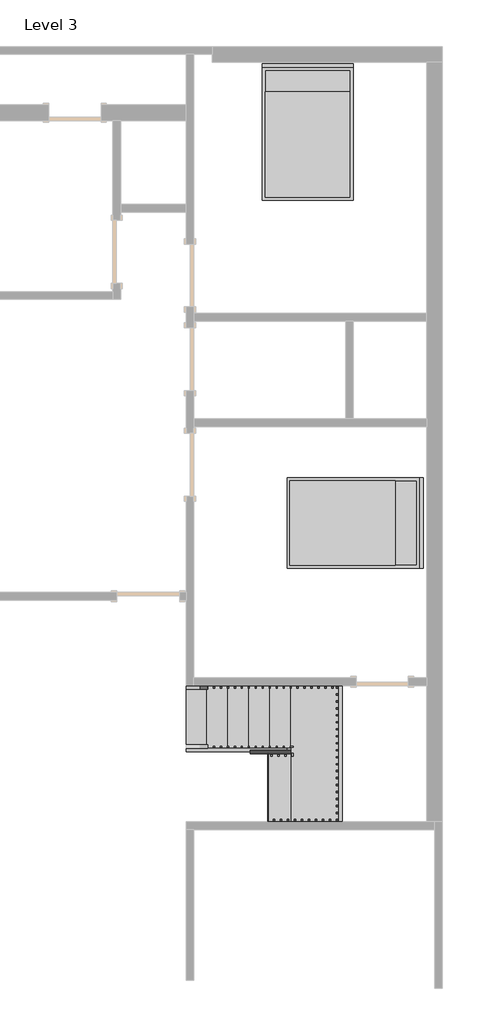
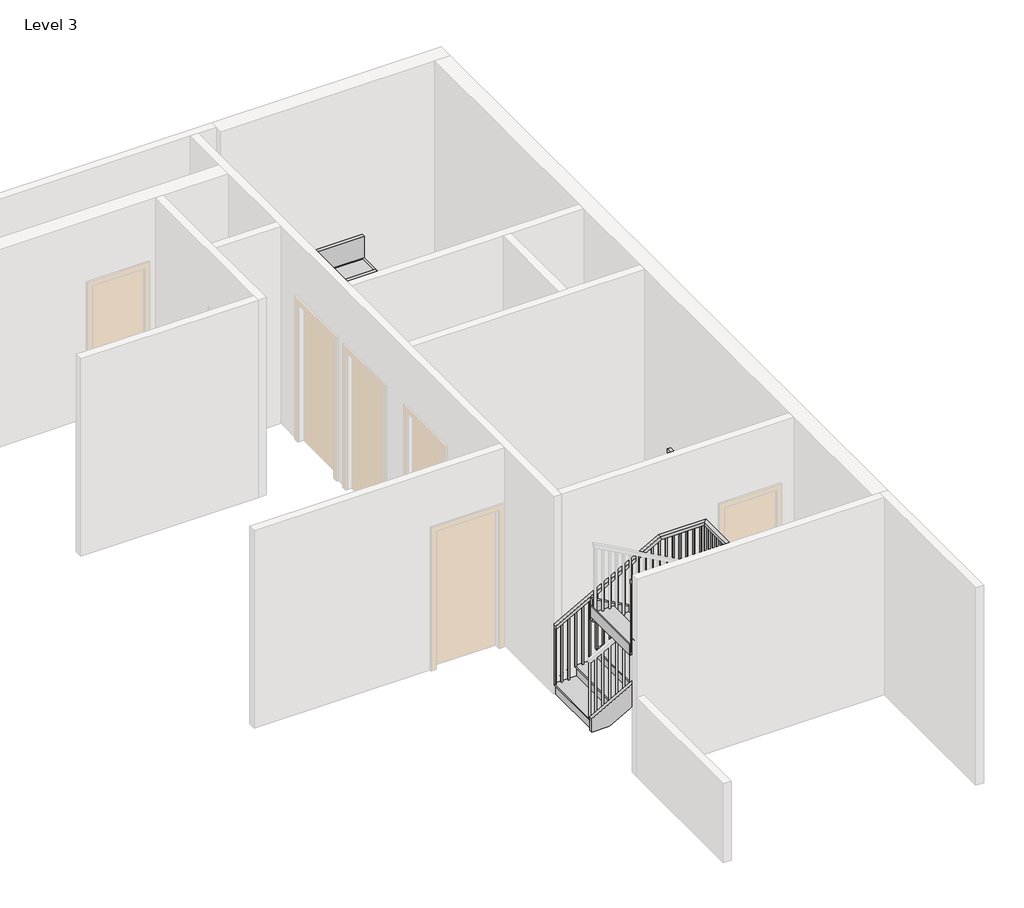
# One storey, part 2 of 2: 6 members, 2 furniture elements, 1 railing, 1 stair flight.
"""IFC4 building model written with IfcOpenShell, lengths in millimetres."""

from ifc_helpers import new_model, si_unit, frame, origin, place, context, project, spatial, polyline, outline, extrude, faceted_brep, transform, mapped, element, save
from components import bed_17739_bed_17739_15c61121, stair_flight_96a85028

model = new_model("IFC4")

# Units and contexts
model_context = context("Model", 3, world=origin())
ifc_project = project(units=[si_unit("LENGTHUNIT", "METRE", prefix="MILLI")], contexts=[model_context])

# Site, building, storey
site = spatial("IfcSite", under=ifc_project)
building = spatial("IfcBuilding", under=site)
storey = spatial("IfcBuildingStorey", under=building, Name="Level 3", Elevation=3200.4)

# Furniture
placement = place(None, origin())
bed_17739_bed_17739_shape = bed_17739_bed_17739_15c61121(model_context)
element("IfcFurniture", 1, ObjectType="Bed_17739 : Bed_17739", at=placement, inside=storey, context=model_context, shape_type="MappedRepresentation", body=[
    mapped(bed_17739_bed_17739_shape, transform((592.6084916, 6126.1935985, 3200.4), x_axis=(1.0, 0.0, 0.0), y_axis=(0.0, 1.0, 0.0), z_axis=(0.0, 0.0, 1.0))),
])
element("IfcFurniture", 2, ObjectType="Bed_17739 : Bed_17739", at=placement, inside=storey, context=model_context, shape_type="MappedRepresentation", body=[
    mapped(bed_17739_bed_17739_shape, transform((1259.3584916, 455.6435985, 3200.4), x_axis=(0.0, -1.0, 0.0), y_axis=(1.0, 0.0, 0.0), z_axis=(0.0, 0.0, 1.0))),
])

# Members
element("IfcMember", 3, ObjectType="Stringer - 2\" Width", at=placement, inside=storey, context=model_context, shape_type="SweptSolid", body=[
    extrude(outline(polyline([(3407.9983948, -1179.0415084), (3200.4, -1179.0415084), (3200.4, -925.0970056), (4292.6, 1040.8629944), (4292.6, 413.241381), (3407.9983948, -1179.0415084)])), frame((0.0, -1912.9064015, 0.0), z_axis=(0.0, 1.0, 0.0), x_axis=(0.0, 0.0, 1.0)), (0.0, 0.0, 1.0), 50.8),
])
element("IfcMember", 4, ObjectType="Stringer - 2\" Width", at=placement, inside=storey, context=model_context, shape_type="SweptSolid", body=[
    extrude(outline(polyline([(1043.4584916, -1862.1064015), (1094.2584916, -1862.1064015), (1094.2584916, -3894.1064015), (1043.4584916, -3894.1064015), (1043.4584916, -1862.1064015)])), frame((0.0, 0.0, 3987.8), z_axis=(0.0, 0.0, 1.0), x_axis=(1.0, 0.0, 0.0)), (0.0, 0.0, 1.0), 304.8),
])
element("IfcMember", 5, ObjectType="Stringer - 2\" Width", at=placement, inside=storey, context=model_context, shape_type="SweptSolid", body=[
    extrude(outline(polyline([(3987.8, 1094.2584916), (4007.720617, 1094.2584916), (5270.6650614, -1179.0415084), (4921.9863873, -1179.0415084), (3987.8, 502.4939888), (3987.8, 1094.2584916)])), frame((0.0, -3944.9064015, 0.0), z_axis=(0.0, 1.0, 0.0), x_axis=(0.0, 0.0, 1.0)), (0.0, 0.0, 1.0), 50.8),
])
element("IfcMember", 6, ObjectType="Stringer - 2\" Width", at=placement, inside=storey, context=model_context, shape_type="SweptSolid", body=[
    extrude(outline(polyline([(3407.9983948, -1179.0415084), (3200.4, -1179.0415084), (3200.4, -925.0970056), (3877.7641651, 294.1584916), (4226.4428392, 294.1584916), (3407.9983948, -1179.0415084)])), frame((0.0, -2878.1064015, 0.0), z_axis=(0.0, 1.0, 0.0), x_axis=(0.0, 0.0, 1.0)), (0.0, 0.0, 1.0), 50.8),
])
element("IfcMember", 7, ObjectType="Stringer - 2\" Width", at=placement, inside=storey, context=model_context, shape_type="SweptSolid", body=[
    extrude(outline(polyline([(294.1584916, -2827.3064015), (344.9584916, -2827.3064015), (344.9584916, -2852.7064015), (294.1584916, -2852.7064015), (294.1584916, -2827.3064015)])), frame((0.0, 0.0, 3987.8), z_axis=(0.0, 0.0, 1.0), x_axis=(1.0, 0.0, 0.0)), (0.0, 0.0, 1.0), 304.8),
])
element("IfcMember", 8, ObjectType="Stringer - 2\" Width", at=placement, inside=storey, context=model_context, shape_type="SweptSolid", body=[
    extrude(outline(polyline([(4075.3197207, 344.9584916), (4423.9983948, 344.9584916), (5270.6650614, -1179.0415084), (4921.9863873, -1179.0415084), (4075.3197207, 344.9584916)])), frame((0.0, -2903.5064015, 0.0), z_axis=(0.0, 1.0, 0.0), x_axis=(0.0, 0.0, 1.0)), (0.0, 0.0, 1.0), 50.8),
])

# Railing
element("IfcRailing", 9, ObjectType="Handrail - Rectangular", at=placement, inside=storey, context=model_context, shape_type="SolidModel", body=[
    faceted_brep([(-1179.0415084, -1912.9064015, 4284.1333333), (-1179.0415084, -1912.9064015, 4226.020221), (-1179.0415084, -1963.7064015, 4226.020221), (-1179.0415084, -1963.7064015, 4284.1333333), (344.9584916, -1912.9064015, 5130.8), (358.1220938, -1912.9064015, 5080.0), (358.1220938, -1963.7064015, 5080.0), (344.9584916, -1963.7064015, 5130.8), (1043.4584916, -1912.9064015, 5130.8), (1043.4584916, -1912.9064015, 5080.0), (992.6584916, -1963.7064015, 5080.0), (992.6584916, -1963.7064015, 5130.8), (1043.4584916, -3894.1064015, 5130.8), (1043.4584916, -3894.1064015, 5080.0), (992.6584916, -3843.3064015, 5080.0), (992.6584916, -3843.3064015, 5130.8), (649.7584916, -3894.1064015, 5130.8), (636.5948894, -3894.1064015, 5080.0), (636.5948894, -3843.3064015, 5080.0), (649.7584916, -3843.3064015, 5130.8), (-1179.0415084, -3894.1064015, 6146.8), (-1179.0415084, -3843.3064015, 6146.8), (-1179.0415084, -3843.3064015, 6088.6868876), (-1179.0415084, -3894.1064015, 6088.6868876)], [[[0, 1, 2, 3]], [[1, 0, 4, 5]], [[2, 1, 5, 6]], [[3, 2, 6, 7]], [[0, 3, 7, 4]], [[5, 4, 8, 9]], [[6, 5, 9, 10]], [[7, 6, 10, 11]], [[4, 7, 11, 8]], [[9, 8, 12, 13]], [[10, 9, 13, 14]], [[11, 10, 14, 15]], [[8, 11, 15, 12]], [[13, 12, 16, 17]], [[14, 13, 17, 18]], [[15, 14, 18, 19]], [[12, 15, 19, 16]], [[20, 21, 22, 23]], [[17, 16, 20, 23]], [[18, 17, 23, 22]], [[19, 18, 22, 21]], [[16, 19, 21, 20]]]),
    extrude(outline(polyline([(6058.7007765, -1125.0665084), (5063.0666667, -1125.0665084), (5063.0666667, -1106.0165084), (6048.1174432, -1106.0165084), (6058.7007765, -1125.0665084)])), frame((0.0, -3878.2314015, 0.0), z_axis=(0.0, 1.0, 0.0), x_axis=(0.0, 0.0, 1.0)), (0.0, 0.0, 1.0), 19.05),
    extrude(outline(polyline([(6002.2563321, -1023.4665084), (5063.0666667, -1023.4665084), (5063.0666667, -1004.4165084), (5991.6729988, -1004.4165084), (6002.2563321, -1023.4665084)])), frame((0.0, -3878.2314015, 0.0), z_axis=(0.0, 1.0, 0.0), x_axis=(0.0, 0.0, 1.0)), (0.0, 0.0, 1.0), 19.05),
    extrude(outline(polyline([(5945.8118876, -921.8665084), (5063.0666667, -921.8665084), (5063.0666667, -902.8165084), (5935.2285543, -902.8165084), (5945.8118876, -921.8665084)])), frame((0.0, -3878.2314015, 0.0), z_axis=(0.0, 1.0, 0.0), x_axis=(0.0, 0.0, 1.0)), (0.0, 0.0, 1.0), 19.05),
    extrude(outline(polyline([(5889.3674432, -820.2665084), (4893.7333333, -820.2665084), (4893.7333333, -801.2165084), (5878.7841099, -801.2165084), (5889.3674432, -820.2665084)])), frame((0.0, -3878.2314015, 0.0), z_axis=(0.0, 1.0, 0.0), x_axis=(0.0, 0.0, 1.0)), (0.0, 0.0, 1.0), 19.05),
    extrude(outline(polyline([(5832.9229988, -718.6665084), (4893.7333333, -718.6665084), (4893.7333333, -699.6165084), (5822.3396654, -699.6165084), (5832.9229988, -718.6665084)])), frame((0.0, -3878.2314015, 0.0), z_axis=(0.0, 1.0, 0.0), x_axis=(0.0, 0.0, 1.0)), (0.0, 0.0, 1.0), 19.05),
    extrude(outline(polyline([(5776.4785543, -617.0665084), (4893.7333333, -617.0665084), (4893.7333333, -598.0165084), (5765.895221, -598.0165084), (5776.4785543, -617.0665084)])), frame((0.0, -3878.2314015, 0.0), z_axis=(0.0, 1.0, 0.0), x_axis=(0.0, 0.0, 1.0)), (0.0, 0.0, 1.0), 19.05),
    extrude(outline(polyline([(5720.0341099, -515.4665084), (4724.4, -515.4665084), (4724.4, -496.4165084), (5709.4507765, -496.4165084), (5720.0341099, -515.4665084)])), frame((0.0, -3878.2314015, 0.0), z_axis=(0.0, 1.0, 0.0), x_axis=(0.0, 0.0, 1.0)), (0.0, 0.0, 1.0), 19.05),
    extrude(outline(polyline([(5663.5896654, -413.8665084), (4724.4, -413.8665084), (4724.4, -394.8165084), (5653.0063321, -394.8165084), (5663.5896654, -413.8665084)])), frame((0.0, -3878.2314015, 0.0), z_axis=(0.0, 1.0, 0.0), x_axis=(0.0, 0.0, 1.0)), (0.0, 0.0, 1.0), 19.05),
    extrude(outline(polyline([(5607.145221, -312.2665084), (4724.4, -312.2665084), (4724.4, -293.2165084), (5596.5618876, -293.2165084), (5607.145221, -312.2665084)])), frame((0.0, -3878.2314015, 0.0), z_axis=(0.0, 1.0, 0.0), x_axis=(0.0, 0.0, 1.0)), (0.0, 0.0, 1.0), 19.05),
    extrude(outline(polyline([(5550.7007765, -210.6665084), (4555.0666667, -210.6665084), (4555.0666667, -191.6165084), (5540.1174432, -191.6165084), (5550.7007765, -210.6665084)])), frame((0.0, -3878.2314015, 0.0), z_axis=(0.0, 1.0, 0.0), x_axis=(0.0, 0.0, 1.0)), (0.0, 0.0, 1.0), 19.05),
    extrude(outline(polyline([(5494.2563321, -109.0665084), (4555.0666667, -109.0665084), (4555.0666667, -90.0165084), (5483.6729988, -90.0165084), (5494.2563321, -109.0665084)])), frame((0.0, -3878.2314015, 0.0), z_axis=(0.0, 1.0, 0.0), x_axis=(0.0, 0.0, 1.0)), (0.0, 0.0, 1.0), 19.05),
    extrude(outline(polyline([(5437.8118876, -7.4665084), (4555.0666667, -7.4665084), (4555.0666667, 11.5834916), (5427.2285543, 11.5834916), (5437.8118876, -7.4665084)])), frame((0.0, -3878.2314015, 0.0), z_axis=(0.0, 1.0, 0.0), x_axis=(0.0, 0.0, 1.0)), (0.0, 0.0, 1.0), 19.05),
    extrude(outline(polyline([(5381.3674432, 94.1334916), (4385.7333333, 94.1334916), (4385.7333333, 113.1834916), (5370.7841099, 113.1834916), (5381.3674432, 94.1334916)])), frame((0.0, -3878.2314015, 0.0), z_axis=(0.0, 1.0, 0.0), x_axis=(0.0, 0.0, 1.0)), (0.0, 0.0, 1.0), 19.05),
    extrude(outline(polyline([(5324.9229988, 195.7334916), (4385.7333333, 195.7334916), (4385.7333333, 214.7834916), (5314.3396654, 214.7834916), (5324.9229988, 195.7334916)])), frame((0.0, -3878.2314015, 0.0), z_axis=(0.0, 1.0, 0.0), x_axis=(0.0, 0.0, 1.0)), (0.0, 0.0, 1.0), 19.05),
    extrude(outline(polyline([(5268.4785543, 297.3334916), (4385.7333333, 297.3334916), (4385.7333333, 316.3834916), (5257.895221, 316.3834916), (5268.4785543, 297.3334916)])), frame((0.0, -3878.2314015, 0.0), z_axis=(0.0, 1.0, 0.0), x_axis=(0.0, 0.0, 1.0)), (0.0, 0.0, 1.0), 19.05),
    extrude(outline(polyline([(5212.0341099, 398.9334916), (4216.4, 398.9334916), (4216.4, 417.9834916), (5201.4507765, 417.9834916), (5212.0341099, 398.9334916)])), frame((0.0, -3878.2314015, 0.0), z_axis=(0.0, 1.0, 0.0), x_axis=(0.0, 0.0, 1.0)), (0.0, 0.0, 1.0), 19.05),
    extrude(outline(polyline([(5155.5896654, 500.5334916), (4216.4, 500.5334916), (4216.4, 519.5834916), (5145.0063321, 519.5834916), (5155.5896654, 500.5334916)])), frame((0.0, -3878.2314015, 0.0), z_axis=(0.0, 1.0, 0.0), x_axis=(0.0, 0.0, 1.0)), (0.0, 0.0, 1.0), 19.05),
    extrude(outline(polyline([(5099.145221, 602.1334916), (4216.4, 602.1334916), (4216.4, 621.1834916), (5088.5618876, 621.1834916), (5099.145221, 602.1334916)])), frame((0.0, -3878.2314015, 0.0), z_axis=(0.0, 1.0, 0.0), x_axis=(0.0, 0.0, 1.0)), (0.0, 0.0, 1.0), 19.05),
    extrude(outline(polyline([(722.7834916, -3878.2314015), (703.7334916, -3878.2314015), (703.7334916, -3859.1814015), (722.7834916, -3859.1814015), (722.7834916, -3878.2314015)])), frame((0.0, 0.0, 4216.4), z_axis=(0.0, 0.0, 1.0), x_axis=(1.0, 0.0, 0.0)), (0.0, 0.0, 1.0), 863.6),
    extrude(outline(polyline([(824.3834916, -3878.2314015), (805.3334916, -3878.2314015), (805.3334916, -3859.1814015), (824.3834916, -3859.1814015), (824.3834916, -3878.2314015)])), frame((0.0, 0.0, 4216.4), z_axis=(0.0, 0.0, 1.0), x_axis=(1.0, 0.0, 0.0)), (0.0, 0.0, 1.0), 863.6),
    extrude(outline(polyline([(925.9834916, -3878.2314015), (906.9334916, -3878.2314015), (906.9334916, -3859.1814015), (925.9834916, -3859.1814015), (925.9834916, -3878.2314015)])), frame((0.0, 0.0, 4216.4), z_axis=(0.0, 0.0, 1.0), x_axis=(1.0, 0.0, 0.0)), (0.0, 0.0, 1.0), 863.6),
    extrude(outline(polyline([(1027.5834916, -3757.5814015), (1027.5834916, -3776.6314015), (1008.5334916, -3776.6314015), (1008.5334916, -3757.5814015), (1027.5834916, -3757.5814015)])), frame((0.0, 0.0, 4216.4), z_axis=(0.0, 0.0, 1.0), x_axis=(1.0, 0.0, 0.0)), (0.0, 0.0, 1.0), 863.6),
    extrude(outline(polyline([(1027.5834916, -3655.9814015), (1027.5834916, -3675.0314015), (1008.5334916, -3675.0314015), (1008.5334916, -3655.9814015), (1027.5834916, -3655.9814015)])), frame((0.0, 0.0, 4216.4), z_axis=(0.0, 0.0, 1.0), x_axis=(1.0, 0.0, 0.0)), (0.0, 0.0, 1.0), 863.6),
    extrude(outline(polyline([(1027.5834916, -3554.3814015), (1027.5834916, -3573.4314015), (1008.5334916, -3573.4314015), (1008.5334916, -3554.3814015), (1027.5834916, -3554.3814015)])), frame((0.0, 0.0, 4216.4), z_axis=(0.0, 0.0, 1.0), x_axis=(1.0, 0.0, 0.0)), (0.0, 0.0, 1.0), 863.6),
    extrude(outline(polyline([(1027.5834916, -3452.7814015), (1027.5834916, -3471.8314015), (1008.5334916, -3471.8314015), (1008.5334916, -3452.7814015), (1027.5834916, -3452.7814015)])), frame((0.0, 0.0, 4216.4), z_axis=(0.0, 0.0, 1.0), x_axis=(1.0, 0.0, 0.0)), (0.0, 0.0, 1.0), 863.6),
    extrude(outline(polyline([(1027.5834916, -3351.1814015), (1027.5834916, -3370.2314015), (1008.5334916, -3370.2314015), (1008.5334916, -3351.1814015), (1027.5834916, -3351.1814015)])), frame((0.0, 0.0, 4216.4), z_axis=(0.0, 0.0, 1.0), x_axis=(1.0, 0.0, 0.0)), (0.0, 0.0, 1.0), 863.6),
    extrude(outline(polyline([(1027.5834916, -3249.5814015), (1027.5834916, -3268.6314015), (1008.5334916, -3268.6314015), (1008.5334916, -3249.5814015), (1027.5834916, -3249.5814015)])), frame((0.0, 0.0, 4216.4), z_axis=(0.0, 0.0, 1.0), x_axis=(1.0, 0.0, 0.0)), (0.0, 0.0, 1.0), 863.6),
    extrude(outline(polyline([(1027.5834916, -3147.9814015), (1027.5834916, -3167.0314015), (1008.5334916, -3167.0314015), (1008.5334916, -3147.9814015), (1027.5834916, -3147.9814015)])), frame((0.0, 0.0, 4216.4), z_axis=(0.0, 0.0, 1.0), x_axis=(1.0, 0.0, 0.0)), (0.0, 0.0, 1.0), 863.6),
    extrude(outline(polyline([(1027.5834916, -3046.3814015), (1027.5834916, -3065.4314015), (1008.5334916, -3065.4314015), (1008.5334916, -3046.3814015), (1027.5834916, -3046.3814015)])), frame((0.0, 0.0, 4216.4), z_axis=(0.0, 0.0, 1.0), x_axis=(1.0, 0.0, 0.0)), (0.0, 0.0, 1.0), 863.6),
    extrude(outline(polyline([(1027.5834916, -2944.7814015), (1027.5834916, -2963.8314015), (1008.5334916, -2963.8314015), (1008.5334916, -2944.7814015), (1027.5834916, -2944.7814015)])), frame((0.0, 0.0, 4216.4), z_axis=(0.0, 0.0, 1.0), x_axis=(1.0, 0.0, 0.0)), (0.0, 0.0, 1.0), 863.6),
    extrude(outline(polyline([(1027.5834916, -2843.1814015), (1027.5834916, -2862.2314015), (1008.5334916, -2862.2314015), (1008.5334916, -2843.1814015), (1027.5834916, -2843.1814015)])), frame((0.0, 0.0, 4216.4), z_axis=(0.0, 0.0, 1.0), x_axis=(1.0, 0.0, 0.0)), (0.0, 0.0, 1.0), 863.6),
    extrude(outline(polyline([(1027.5834916, -2741.5814015), (1027.5834916, -2760.6314015), (1008.5334916, -2760.6314015), (1008.5334916, -2741.5814015), (1027.5834916, -2741.5814015)])), frame((0.0, 0.0, 4216.4), z_axis=(0.0, 0.0, 1.0), x_axis=(1.0, 0.0, 0.0)), (0.0, 0.0, 1.0), 863.6),
    extrude(outline(polyline([(1027.5834916, -2639.9814015), (1027.5834916, -2659.0314015), (1008.5334916, -2659.0314015), (1008.5334916, -2639.9814015), (1027.5834916, -2639.9814015)])), frame((0.0, 0.0, 4216.4), z_axis=(0.0, 0.0, 1.0), x_axis=(1.0, 0.0, 0.0)), (0.0, 0.0, 1.0), 863.6),
    extrude(outline(polyline([(1027.5834916, -2538.3814015), (1027.5834916, -2557.4314015), (1008.5334916, -2557.4314015), (1008.5334916, -2538.3814015), (1027.5834916, -2538.3814015)])), frame((0.0, 0.0, 4216.4), z_axis=(0.0, 0.0, 1.0), x_axis=(1.0, 0.0, 0.0)), (0.0, 0.0, 1.0), 863.6),
    extrude(outline(polyline([(1027.5834916, -2436.7814015), (1027.5834916, -2455.8314015), (1008.5334916, -2455.8314015), (1008.5334916, -2436.7814015), (1027.5834916, -2436.7814015)])), frame((0.0, 0.0, 4216.4), z_axis=(0.0, 0.0, 1.0), x_axis=(1.0, 0.0, 0.0)), (0.0, 0.0, 1.0), 863.6),
    extrude(outline(polyline([(1027.5834916, -2335.1814015), (1027.5834916, -2354.2314015), (1008.5334916, -2354.2314015), (1008.5334916, -2335.1814015), (1027.5834916, -2335.1814015)])), frame((0.0, 0.0, 4216.4), z_axis=(0.0, 0.0, 1.0), x_axis=(1.0, 0.0, 0.0)), (0.0, 0.0, 1.0), 863.6),
    extrude(outline(polyline([(1027.5834916, -2233.5814015), (1027.5834916, -2252.6314015), (1008.5334916, -2252.6314015), (1008.5334916, -2233.5814015), (1027.5834916, -2233.5814015)])), frame((0.0, 0.0, 4216.4), z_axis=(0.0, 0.0, 1.0), x_axis=(1.0, 0.0, 0.0)), (0.0, 0.0, 1.0), 863.6),
    extrude(outline(polyline([(1027.5834916, -2131.9814015), (1027.5834916, -2151.0314015), (1008.5334916, -2151.0314015), (1008.5334916, -2131.9814015), (1027.5834916, -2131.9814015)])), frame((0.0, 0.0, 4216.4), z_axis=(0.0, 0.0, 1.0), x_axis=(1.0, 0.0, 0.0)), (0.0, 0.0, 1.0), 863.6),
    extrude(outline(polyline([(1027.5834916, -2030.3814015), (1027.5834916, -2049.4314015), (1008.5334916, -2049.4314015), (1008.5334916, -2030.3814015), (1027.5834916, -2030.3814015)])), frame((0.0, 0.0, 4216.4), z_axis=(0.0, 0.0, 1.0), x_axis=(1.0, 0.0, 0.0)), (0.0, 0.0, 1.0), 863.6),
    extrude(outline(polyline([(945.0334916, -1928.7814015), (964.0834916, -1928.7814015), (964.0834916, -1947.8314015), (945.0334916, -1947.8314015), (945.0334916, -1928.7814015)])), frame((0.0, 0.0, 4216.4), z_axis=(0.0, 0.0, 1.0), x_axis=(1.0, 0.0, 0.0)), (0.0, 0.0, 1.0), 863.6),
    extrude(outline(polyline([(843.4334916, -1928.7814015), (862.4834916, -1928.7814015), (862.4834916, -1947.8314015), (843.4334916, -1947.8314015), (843.4334916, -1928.7814015)])), frame((0.0, 0.0, 4216.4), z_axis=(0.0, 0.0, 1.0), x_axis=(1.0, 0.0, 0.0)), (0.0, 0.0, 1.0), 863.6),
    extrude(outline(polyline([(741.8334916, -1928.7814015), (760.8834916, -1928.7814015), (760.8834916, -1947.8314015), (741.8334916, -1947.8314015), (741.8334916, -1928.7814015)])), frame((0.0, 0.0, 4216.4), z_axis=(0.0, 0.0, 1.0), x_axis=(1.0, 0.0, 0.0)), (0.0, 0.0, 1.0), 863.6),
    extrude(outline(polyline([(640.2334916, -1928.7814015), (659.2834916, -1928.7814015), (659.2834916, -1947.8314015), (640.2334916, -1947.8314015), (640.2334916, -1928.7814015)])), frame((0.0, 0.0, 4216.4), z_axis=(0.0, 0.0, 1.0), x_axis=(1.0, 0.0, 0.0)), (0.0, 0.0, 1.0), 863.6),
    extrude(outline(polyline([(538.6334916, -1928.7814015), (557.6834916, -1928.7814015), (557.6834916, -1947.8314015), (538.6334916, -1947.8314015), (538.6334916, -1928.7814015)])), frame((0.0, 0.0, 4216.4), z_axis=(0.0, 0.0, 1.0), x_axis=(1.0, 0.0, 0.0)), (0.0, 0.0, 1.0), 863.6),
    extrude(outline(polyline([(437.0334916, -1928.7814015), (456.0834916, -1928.7814015), (456.0834916, -1947.8314015), (437.0334916, -1947.8314015), (437.0334916, -1928.7814015)])), frame((0.0, 0.0, 4216.4), z_axis=(0.0, 0.0, 1.0), x_axis=(1.0, 0.0, 0.0)), (0.0, 0.0, 1.0), 863.6),
    extrude(outline(polyline([(5067.395221, 335.4334916), (4216.4, 335.4334916), (4216.4, 354.4834916), (5077.9785543, 354.4834916), (5067.395221, 335.4334916)])), frame((0.0, -1947.8314015, 0.0), z_axis=(0.0, 1.0, 0.0), x_axis=(0.0, 0.0, 1.0)), (0.0, 0.0, 1.0), 19.05),
    extrude(outline(polyline([(5010.9507765, 233.8334916), (4047.0666667, 233.8334916), (4047.0666667, 252.8834916), (5021.5341099, 252.8834916), (5010.9507765, 233.8334916)])), frame((0.0, -1947.8314015, 0.0), z_axis=(0.0, 1.0, 0.0), x_axis=(0.0, 0.0, 1.0)), (0.0, 0.0, 1.0), 19.05),
    extrude(outline(polyline([(4954.5063321, 132.2334916), (4047.0666667, 132.2334916), (4047.0666667, 151.2834916), (4965.0896654, 151.2834916), (4954.5063321, 132.2334916)])), frame((0.0, -1947.8314015, 0.0), z_axis=(0.0, 1.0, 0.0), x_axis=(0.0, 0.0, 1.0)), (0.0, 0.0, 1.0), 19.05),
    extrude(outline(polyline([(4898.0618876, 30.6334916), (4047.0666667, 30.6334916), (4047.0666667, 49.6834916), (4908.645221, 49.6834916), (4898.0618876, 30.6334916)])), frame((0.0, -1947.8314015, 0.0), z_axis=(0.0, 1.0, 0.0), x_axis=(0.0, 0.0, 1.0)), (0.0, 0.0, 1.0), 19.05),
    extrude(outline(polyline([(4841.6174432, -70.9665084), (3877.7333333, -70.9665084), (3877.7333333, -51.9165084), (4852.2007765, -51.9165084), (4841.6174432, -70.9665084)])), frame((0.0, -1947.8314015, 0.0), z_axis=(0.0, 1.0, 0.0), x_axis=(0.0, 0.0, 1.0)), (0.0, 0.0, 1.0), 19.05),
    extrude(outline(polyline([(4785.1729988, -172.5665084), (3877.7333333, -172.5665084), (3877.7333333, -153.5165084), (4795.7563321, -153.5165084), (4785.1729988, -172.5665084)])), frame((0.0, -1947.8314015, 0.0), z_axis=(0.0, 1.0, 0.0), x_axis=(0.0, 0.0, 1.0)), (0.0, 0.0, 1.0), 19.05),
    extrude(outline(polyline([(4728.7285543, -274.1665084), (3877.7333333, -274.1665084), (3877.7333333, -255.1165084), (4739.3118876, -255.1165084), (4728.7285543, -274.1665084)])), frame((0.0, -1947.8314015, 0.0), z_axis=(0.0, 1.0, 0.0), x_axis=(0.0, 0.0, 1.0)), (0.0, 0.0, 1.0), 19.05),
    extrude(outline(polyline([(4672.2841099, -375.7665084), (3708.4, -375.7665084), (3708.4, -356.7165084), (4682.8674432, -356.7165084), (4672.2841099, -375.7665084)])), frame((0.0, -1947.8314015, 0.0), z_axis=(0.0, 1.0, 0.0), x_axis=(0.0, 0.0, 1.0)), (0.0, 0.0, 1.0), 19.05),
    extrude(outline(polyline([(4615.8396654, -477.3665084), (3708.4, -477.3665084), (3708.4, -458.3165084), (4626.4229988, -458.3165084), (4615.8396654, -477.3665084)])), frame((0.0, -1947.8314015, 0.0), z_axis=(0.0, 1.0, 0.0), x_axis=(0.0, 0.0, 1.0)), (0.0, 0.0, 1.0), 19.05),
    extrude(outline(polyline([(4559.395221, -578.9665084), (3708.4, -578.9665084), (3708.4, -559.9165084), (4569.9785543, -559.9165084), (4559.395221, -578.9665084)])), frame((0.0, -1947.8314015, 0.0), z_axis=(0.0, 1.0, 0.0), x_axis=(0.0, 0.0, 1.0)), (0.0, 0.0, 1.0), 19.05),
    extrude(outline(polyline([(4502.9507765, -680.5665084), (3539.0666667, -680.5665084), (3539.0666667, -661.5165084), (4513.5341099, -661.5165084), (4502.9507765, -680.5665084)])), frame((0.0, -1947.8314015, 0.0), z_axis=(0.0, 1.0, 0.0), x_axis=(0.0, 0.0, 1.0)), (0.0, 0.0, 1.0), 19.05),
    extrude(outline(polyline([(4446.5063321, -782.1665084), (3539.0666667, -782.1665084), (3539.0666667, -763.1165084), (4457.0896654, -763.1165084), (4446.5063321, -782.1665084)])), frame((0.0, -1947.8314015, 0.0), z_axis=(0.0, 1.0, 0.0), x_axis=(0.0, 0.0, 1.0)), (0.0, 0.0, 1.0), 19.05),
    extrude(outline(polyline([(4390.0618876, -883.7665084), (3539.0666667, -883.7665084), (3539.0666667, -864.7165084), (4400.645221, -864.7165084), (4390.0618876, -883.7665084)])), frame((0.0, -1947.8314015, 0.0), z_axis=(0.0, 1.0, 0.0), x_axis=(0.0, 0.0, 1.0)), (0.0, 0.0, 1.0), 19.05),
    extrude(outline(polyline([(4333.6174432, -985.3665084), (3369.7333333, -985.3665084), (3369.7333333, -966.3165084), (4344.2007765, -966.3165084), (4333.6174432, -985.3665084)])), frame((0.0, -1947.8314015, 0.0), z_axis=(0.0, 1.0, 0.0), x_axis=(0.0, 0.0, 1.0)), (0.0, 0.0, 1.0), 19.05),
    extrude(outline(polyline([(4277.1729988, -1086.9665084), (3369.7333333, -1086.9665084), (3369.7333333, -1067.9165084), (4287.7563321, -1067.9165084), (4277.1729988, -1086.9665084)])), frame((0.0, -1947.8314015, 0.0), z_axis=(0.0, 1.0, 0.0), x_axis=(0.0, 0.0, 1.0)), (0.0, 0.0, 1.0), 19.05),
    extrude(outline(polyline([(1027.5834916, -3859.1814015), (1027.5834916, -3878.2314015), (1008.5334916, -3878.2314015), (1008.5334916, -3859.1814015), (1027.5834916, -3859.1814015)])), frame((0.0, 0.0, 4216.4), z_axis=(0.0, 0.0, 1.0), x_axis=(1.0, 0.0, 0.0)), (0.0, 0.0, 1.0), 863.6),
    extrude(outline(polyline([(1008.5334916, -1928.7814015), (1027.5834916, -1928.7814015), (1027.5834916, -1947.8314015), (1008.5334916, -1947.8314015), (1008.5334916, -1928.7814015)])), frame((0.0, 0.0, 4216.4), z_axis=(0.0, 0.0, 1.0), x_axis=(1.0, 0.0, 0.0)), (0.0, 0.0, 1.0), 863.6),
    extrude(outline(polyline([(6088.6868876, -1179.0415084), (5063.0666667, -1179.0415084), (5063.0666667, -1159.9915084), (6078.1035543, -1159.9915084), (6088.6868876, -1179.0415084)])), frame((0.0, -3878.2314015, 0.0), z_axis=(0.0, 1.0, 0.0), x_axis=(0.0, 0.0, 1.0)), (0.0, 0.0, 1.0), 19.05),
    extrude(outline(polyline([(4226.020221, -1179.0415084), (3369.7333333, -1179.0415084), (3369.7333333, -1159.9915084), (4236.6035543, -1159.9915084), (4226.020221, -1179.0415084)])), frame((0.0, -1947.8314015, 0.0), z_axis=(0.0, 1.0, 0.0), x_axis=(0.0, 0.0, 1.0)), (0.0, 0.0, 1.0), 19.05),
])

# Stair flight
stair_flight_shape = stair_flight_96a85028(model_context)
element("IfcStairFlight", 10, ObjectType="2\" Tread 1\" Nosing 1/4\" Riser", at=placement, inside=storey, context=model_context, shape_type="MappedRepresentation", body=[
    mapped(stair_flight_shape, transform((0.0, 0.0, 0.0), x_axis=(1.0, 0.0, 0.0), y_axis=(0.0, 1.0, 0.0), z_axis=(0.0, 0.0, 1.0))),
])

save(model, "model.ifc")

# Revit data of these elements
# Type "Bed_17739 : Bed_17739"
#   Default Elevation = 0
# Type "Handrail - Rectangular"
#   Assembly Code = "C2010400"
#   built-in parameter 1008612 = 0.0416667 (stored number, unit not read)
#   built-in parameter 1008611 = 0.0416667 (stored number, unit not read)
#   built-in parameter 1008609 = 0.333333 (stored number, unit not read)
#   built-in parameter 1008604 = 0.166667 (stored number, unit not read)
#   built-in parameter 1008603 = 0.166667 (stored number, unit not read)
#   Railing Height = 3' - 0"
#   built-in parameter 1008630 = 2
#   built-in parameter 1008610 = 2
#   built-in parameter 1008618 = Baluster - Square : 3/4"
# Elements 1, 2 (IfcFurniture, "Bed_17739 : Bed_17739")
#   Phase Created = New Construction
#   Materials on its faces: "legs", "sheets", "bed frame", "Blanket"
# Elements 3, 4, 5, 6, 7, 8 (IfcMember, "Stringer - 2\" Width")
#   Phase Created = New Construction
# Element 9 (IfcRailing, "Handrail - Rectangular")
#   Phase Created = New Construction
# Element 10 (IfcStairFlight, "2\" Tread 1\" Nosing 1/4\" Riser")
#   Phase Created = New Construction
# Materials
#   "legs": colour RGB 90 73 37, transparency 0, Cost = 0
#   "sheets": colour RGB 200 195 176, transparency 0, Cost = 0
#   "bed frame": colour RGB 90 73 37, transparency 0, Cost = 0
#   "Blanket": class "System", colour RGB 59 0 1, transparency 0, Cost = 0
